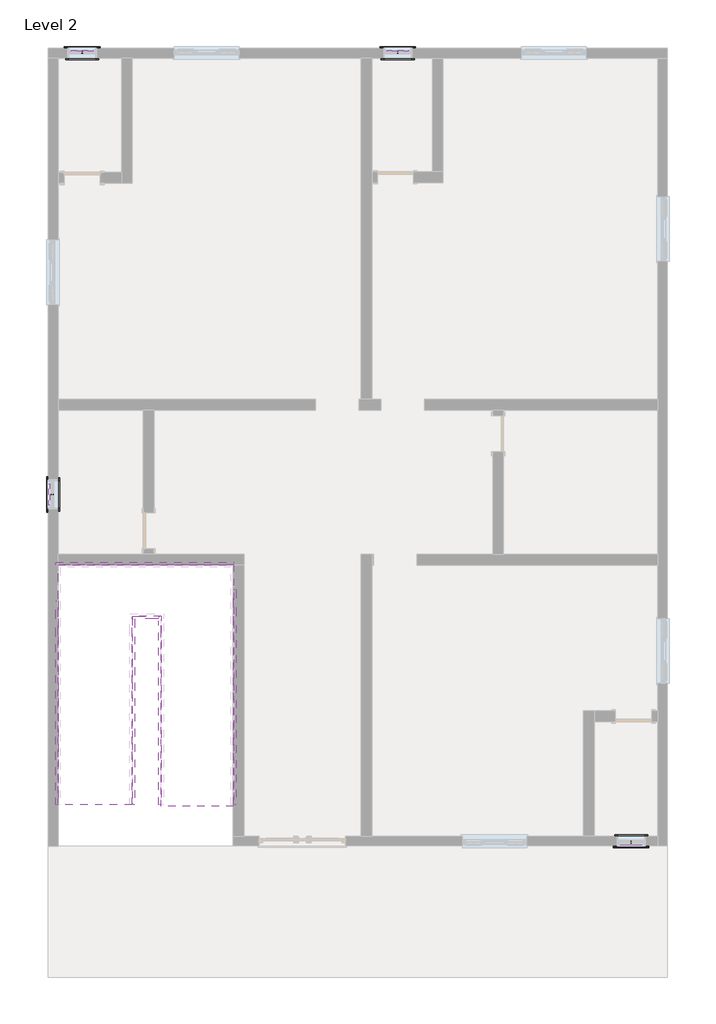
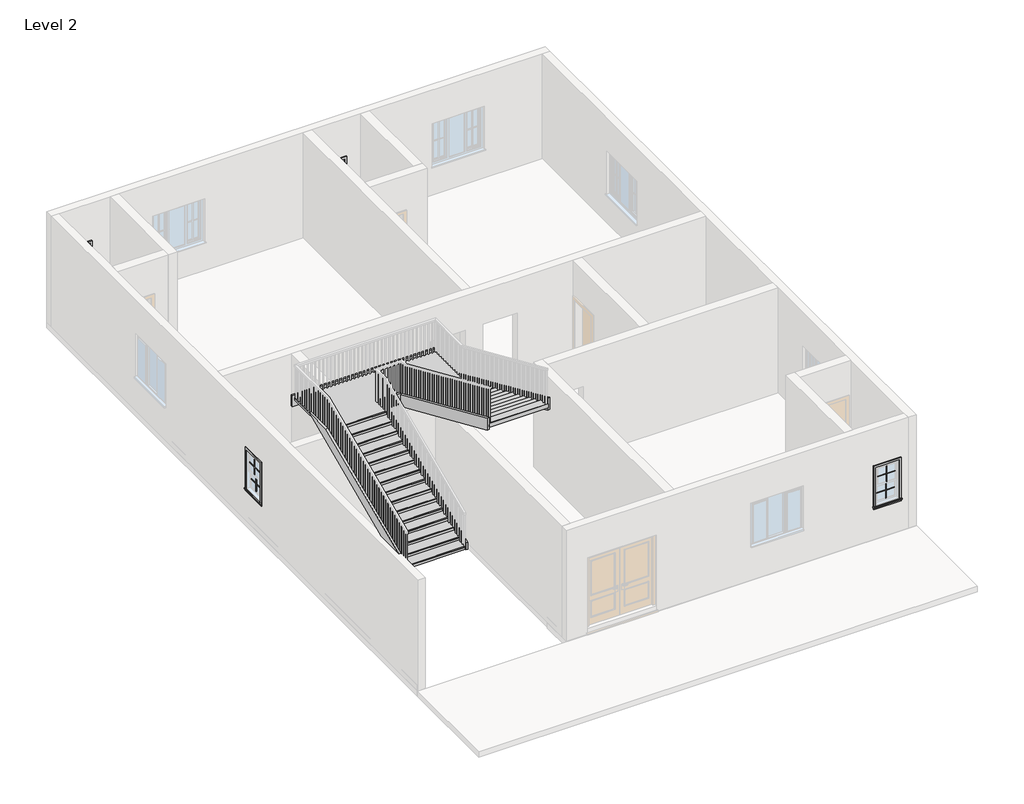
# One storey, part 4 of 4: 16 proxies, 6 members, 1 stair flight.
"""IFC4 building model written with IfcOpenShell, lengths in millimetres."""

from ifc_helpers import new_model, si_unit, frame, origin, place, context, project, spatial, polyline, outline, extrude, transform, mapped, element, save
from components import muntin_pattern_2x2_muntin_pattern_2x2_eba6c5fb, trim_window_exterior_flat_with_sill_278e6a94, trim_window_interior_flat_picture_frame_e9fd5f45, stair_flight_371d2c9c

model = new_model("IFC4")

# Units and contexts
model_context = context("Model", 3, world=origin())
ifc_project = project(units=[si_unit("LENGTHUNIT", "METRE", prefix="MILLI")], contexts=[model_context])

# Site, building, storey
site = spatial("IfcSite", under=ifc_project)
building = spatial("IfcBuilding", under=site)
storey = spatial("IfcBuildingStorey", under=building, Name="Level 2", Elevation=3048.0)

# Proxies
placement = place(None, origin())
muntin_pattern_2x2_muntin_pattern_2x2_shape = muntin_pattern_2x2_muntin_pattern_2x2_eba6c5fb(model_context)
element("IfcBuildingElementProxy", 1, Name="Muntin Pattern_2x2 : Muntin Pattern_2x2", ObjectType="Muntin Pattern_2x2 : Muntin Pattern_2x2", at=placement, inside=storey, context=model_context, shape_type="MappedRepresentation", body=[
    mapped(muntin_pattern_2x2_muntin_pattern_2x2_shape, transform((-7722.7165084, -455.2217109, 4518.025), x_axis=(0.0, 1.0, 0.0), y_axis=(-1.0, 0.0, 0.0), z_axis=(0.0, 0.0, 1.0))),
])
element("IfcBuildingElementProxy", 2, Name="Muntin Pattern_2x2 : Muntin Pattern_2x2", ObjectType="Muntin Pattern_2x2 : Muntin Pattern_2x2", at=placement, inside=storey, context=model_context, shape_type="MappedRepresentation", body=[
    mapped(muntin_pattern_2x2_muntin_pattern_2x2_shape, transform((-7678.2665084, -455.2217109, 4038.6), x_axis=(0.0, 1.0, 0.0), y_axis=(-1.0, 0.0, 0.0), z_axis=(0.0, 0.0, 1.0))),
])
element("IfcBuildingElementProxy", 3, Name="Muntin Pattern_2x2 : Muntin Pattern_2x2", ObjectType="Muntin Pattern_2x2 : Muntin Pattern_2x2", at=placement, inside=storey, context=model_context, shape_type="MappedRepresentation", body=[
    mapped(muntin_pattern_2x2_muntin_pattern_2x2_shape, transform((-7046.4415084, 8872.5685985, 4518.025), x_axis=(1.0, 0.0, 0.0), y_axis=(0.0, 1.0, 0.0), z_axis=(0.0, 0.0, 1.0))),
])
element("IfcBuildingElementProxy", 4, Name="Muntin Pattern_2x2 : Muntin Pattern_2x2", ObjectType="Muntin Pattern_2x2 : Muntin Pattern_2x2", at=placement, inside=storey, context=model_context, shape_type="MappedRepresentation", body=[
    mapped(muntin_pattern_2x2_muntin_pattern_2x2_shape, transform((-7046.4415084, 8828.1185985, 4038.6), x_axis=(1.0, 0.0, 0.0), y_axis=(0.0, 1.0, 0.0), z_axis=(0.0, 0.0, 1.0))),
])
element("IfcBuildingElementProxy", 5, Name="Muntin Pattern_2x2 : Muntin Pattern_2x2", ObjectType="Muntin Pattern_2x2 : Muntin Pattern_2x2", at=placement, inside=storey, context=model_context, shape_type="MappedRepresentation", body=[
    mapped(muntin_pattern_2x2_muntin_pattern_2x2_shape, transform((-417.0415084, 8872.5685985, 4518.025), x_axis=(1.0, 0.0, 0.0), y_axis=(0.0, 1.0, 0.0), z_axis=(0.0, 0.0, 1.0))),
])
element("IfcBuildingElementProxy", 6, Name="Muntin Pattern_2x2 : Muntin Pattern_2x2", ObjectType="Muntin Pattern_2x2 : Muntin Pattern_2x2", at=placement, inside=storey, context=model_context, shape_type="MappedRepresentation", body=[
    mapped(muntin_pattern_2x2_muntin_pattern_2x2_shape, transform((-417.0415084, 8828.1185985, 4038.6), x_axis=(1.0, 0.0, 0.0), y_axis=(0.0, 1.0, 0.0), z_axis=(0.0, 0.0, 1.0))),
])
element("IfcBuildingElementProxy", 7, Name="Muntin Pattern_2x2 : Muntin Pattern_2x2", ObjectType="Muntin Pattern_2x2 : Muntin Pattern_2x2", at=placement, inside=storey, context=model_context, shape_type="MappedRepresentation", body=[
    mapped(muntin_pattern_2x2_muntin_pattern_2x2_shape, transform((4485.1584916, -7796.1814015, 4518.025), x_axis=(-1.0, 0.0, 0.0), y_axis=(0.0, -1.0, 0.0), z_axis=(0.0, 0.0, 1.0))),
])
element("IfcBuildingElementProxy", 8, Name="Muntin Pattern_2x2 : Muntin Pattern_2x2", ObjectType="Muntin Pattern_2x2 : Muntin Pattern_2x2", at=placement, inside=storey, context=model_context, shape_type="MappedRepresentation", body=[
    mapped(muntin_pattern_2x2_muntin_pattern_2x2_shape, transform((4485.1584916, -7751.7314015, 4038.6), x_axis=(-1.0, 0.0, 0.0), y_axis=(0.0, -1.0, 0.0), z_axis=(0.0, 0.0, 1.0))),
])
trim_window_exterior_flat_with_sill_shape = trim_window_exterior_flat_with_sill_278e6a94(model_context)
element("IfcBuildingElementProxy", 9, Name="Trim-Window-Exterior-Flat : with Sill", ObjectType="Trim-Window-Exterior-Flat : with Sill", at=placement, inside=storey, context=model_context, shape_type="MappedRepresentation", body=[
    mapped(trim_window_exterior_flat_with_sill_shape, transform((-7757.6415084, -455.2217109, 5029.2), x_axis=(0.0, -1.0, 0.0), y_axis=(0.0, 0.0, 1.0), z_axis=(-1.0, 0.0, 0.0))),
])
element("IfcBuildingElementProxy", 10, Name="Trim-Window-Exterior-Flat : with Sill", ObjectType="Trim-Window-Exterior-Flat : with Sill", at=placement, inside=storey, context=model_context, shape_type="MappedRepresentation", body=[
    mapped(trim_window_exterior_flat_with_sill_shape, transform((-7046.4415084, 8907.4935985, 5029.2), x_axis=(-1.0, 0.0, 0.0), y_axis=(0.0, 0.0, 1.0), z_axis=(0.0, 1.0, 0.0))),
])
element("IfcBuildingElementProxy", 11, Name="Trim-Window-Exterior-Flat : with Sill", ObjectType="Trim-Window-Exterior-Flat : with Sill", at=placement, inside=storey, context=model_context, shape_type="MappedRepresentation", body=[
    mapped(trim_window_exterior_flat_with_sill_shape, transform((-417.0415084, 8907.4935985, 5029.2), x_axis=(-1.0, 0.0, 0.0), y_axis=(0.0, 0.0, 1.0), z_axis=(0.0, 1.0, 0.0))),
])
element("IfcBuildingElementProxy", 12, Name="Trim-Window-Exterior-Flat : with Sill", ObjectType="Trim-Window-Exterior-Flat : with Sill", at=placement, inside=storey, context=model_context, shape_type="MappedRepresentation", body=[
    mapped(trim_window_exterior_flat_with_sill_shape, transform((4485.1584916, -7831.1064015, 5029.2), x_axis=(1.0, 0.0, 0.0), y_axis=(0.0, 0.0, 1.0), z_axis=(0.0, -1.0, 0.0))),
])
trim_window_interior_flat_picture_frame_shape = trim_window_interior_flat_picture_frame_e9fd5f45(model_context)
element("IfcBuildingElementProxy", 13, Name="Trim-Window-Interior-Flat : Picture Frame", ObjectType="Trim-Window-Interior-Flat : Picture Frame", at=placement, inside=storey, context=model_context, shape_type="MappedRepresentation", body=[
    mapped(trim_window_interior_flat_picture_frame_shape, transform((-7554.4415084, -455.2217109, 5029.2), x_axis=(0.0, 1.0, 0.0), y_axis=(0.0, 0.0, 1.0), z_axis=(1.0, 0.0, 0.0))),
])
element("IfcBuildingElementProxy", 14, Name="Trim-Window-Interior-Flat : Picture Frame", ObjectType="Trim-Window-Interior-Flat : Picture Frame", at=placement, inside=storey, context=model_context, shape_type="MappedRepresentation", body=[
    mapped(trim_window_interior_flat_picture_frame_shape, transform((-7046.4415084, 8704.2935985, 5029.2), x_axis=(1.0, 0.0, 0.0), y_axis=(0.0, 0.0, 1.0), z_axis=(0.0, -1.0, 0.0))),
])
element("IfcBuildingElementProxy", 15, Name="Trim-Window-Interior-Flat : Picture Frame", ObjectType="Trim-Window-Interior-Flat : Picture Frame", at=placement, inside=storey, context=model_context, shape_type="MappedRepresentation", body=[
    mapped(trim_window_interior_flat_picture_frame_shape, transform((-417.0415084, 8704.2935985, 5029.2), x_axis=(1.0, 0.0, 0.0), y_axis=(0.0, 0.0, 1.0), z_axis=(0.0, -1.0, 0.0))),
])
element("IfcBuildingElementProxy", 16, Name="Trim-Window-Interior-Flat : Picture Frame", ObjectType="Trim-Window-Interior-Flat : Picture Frame", at=placement, inside=storey, context=model_context, shape_type="MappedRepresentation", body=[
    mapped(trim_window_interior_flat_picture_frame_shape, transform((4485.1584916, -7627.9064015, 5029.2), x_axis=(-1.0, 0.0, 0.0), y_axis=(0.0, 0.0, 1.0), z_axis=(0.0, 1.0, 0.0))),
])

# Members
element("IfcMember", 17, ObjectType="Stringer - 2\" Width", at=placement, inside=storey, context=model_context, shape_type="SweptSolid", body=[
    extrude(outline(polyline([(-6973.0610642, 5791.2), (-6973.0610642, 5990.0550815), (-3441.822613, 7543.8), (-2685.0041973, 7543.8), (-6668.1860155, 5791.2), (-6973.0610642, 5791.2)])), frame((-7605.2415084, 0.0, 0.0), z_axis=(1.0, 0.0, 0.0), x_axis=(0.0, 1.0, 0.0)), (0.0, 0.0, 1.0), 50.8),
])
element("IfcMember", 18, ObjectType="Stringer - 2\" Width", at=placement, inside=storey, context=model_context, shape_type="SweptSolid", body=[
    extrude(outline(polyline([(-7605.2415084, -1928.4217109), (-7605.2415084, -1877.6217109), (-3866.3290366, -1877.6217109), (-3866.3290366, -1928.4217109), (-7605.2415084, -1928.4217109)])), frame((0.0, 0.0, 7239.0), z_axis=(0.0, 0.0, 1.0), x_axis=(1.0, 0.0, 0.0)), (0.0, 0.0, 1.0), 304.8),
])
element("IfcMember", 19, ObjectType="Stringer - 2\" Width", at=placement, inside=storey, context=model_context, shape_type="SweptSolid", body=[
    extrude(outline(polyline([(-3202.3906584, 7239.0), (-6973.0610642, 8898.0949786), (-6973.0610642, 9231.0950815), (-2445.5722427, 7239.0), (-3202.3906584, 7239.0)])), frame((-3866.3290366, 0.0, 0.0), z_axis=(1.0, 0.0, 0.0), x_axis=(0.0, 1.0, 0.0)), (0.0, 0.0, 1.0), 50.8),
])
element("IfcMember", 20, ObjectType="Stringer - 2\" Width", at=placement, inside=storey, context=model_context, shape_type="SweptSolid", body=[
    extrude(outline(polyline([(-6973.0610642, 5791.2), (-6973.0610642, 5990.0550815), (-3441.822613, 7543.8), (-3061.4610642, 7543.8), (-3061.4610642, 7378.1589786), (-6668.1860155, 5791.2), (-6973.0610642, 5791.2)])), frame((-5999.9290366, 0.0, 0.0), z_axis=(1.0, 0.0, 0.0), x_axis=(0.0, 1.0, 0.0)), (0.0, 0.0, 1.0), 50.8),
])
element("IfcMember", 21, ObjectType="Stringer - 2\" Width", at=placement, inside=storey, context=model_context, shape_type="SweptSolid", body=[
    extrude(outline(polyline([(-5999.9290366, -3061.4610642), (-5999.9290366, -3010.6610642), (-5441.1290366, -3010.6610642), (-5441.1290366, -3061.4610642), (-5999.9290366, -3061.4610642)])), frame((0.0, 0.0, 7239.0), z_axis=(0.0, 0.0, 1.0), x_axis=(1.0, 0.0, 0.0)), (0.0, 0.0, 1.0), 304.8),
])
element("IfcMember", 22, ObjectType="Stringer - 2\" Width", at=placement, inside=storey, context=model_context, shape_type="SweptSolid", body=[
    extrude(outline(polyline([(-3010.6610642, 7487.6390815), (-3010.6610642, 7239.0), (-3202.3906584, 7239.0), (-6973.0610642, 8898.0949786), (-6973.0610642, 9231.0950815), (-3010.6610642, 7487.6390815)])), frame((-5441.1290366, 0.0, 0.0), z_axis=(1.0, 0.0, 0.0), x_axis=(0.0, 1.0, 0.0)), (0.0, 0.0, 1.0), 50.8),
])

# Stair flight
stair_flight_shape = stair_flight_371d2c9c(model_context)
element("IfcStairFlight", 23, ObjectType="2\" Tread 1\" Nosing 1/4\" Riser", at=placement, inside=storey, context=model_context, shape_type="MappedRepresentation", body=[
    mapped(stair_flight_shape, transform((0.0, 0.0, 0.0), x_axis=(1.0, 0.0, 0.0), y_axis=(0.0, 1.0, 0.0), z_axis=(0.0, 0.0, 1.0))),
])

save(model, "model.ifc")

# Revit data of these elements
# Type "Muntin Pattern_2x2 : Muntin Pattern_2x2"
#   Width [instance default] = 4' - 0"
#   Thickness = 0' - 0 1/2"
#   Height [instance default] = 4' - 0"
#   Distance = 0' - 0 3/4"
#   Interior Material [instance default] = none
#   Exterior Material [instance default] = none
#   Default Elevation = 0
# Type "Trim-Window-Exterior-Flat : with Sill"
#   Trim Width = 0' - 2 1/4"
#   Trim Thickness_Picture Frame = 0' - 1 1/4"
#   Trim Thickness_with Sill = 0' - 0 3/4"
#   Sill Thickness = 0' - 1 1/4"
#   Opening Width [instance default] = 2' - 0"
#   Opening Height [instance default] = 3' - 0"
#   Default Elevation = 4' - 0"
#   Sill = yes
#   Picture Frame = no
#   Trim Material [instance default] = none
# Type "Trim-Window-Interior-Flat : Picture Frame"
#   Trim Thickness_Picture Frame = 0' - 1 1/4"
#   Trim Width = 0' - 2 1/4"
#   Trim Thickness_with Sill = 0' - 0 3/4"
#   Sill Thickness = 0' - 1 1/4"
#   Opening Width [instance default] = 2' - 0"
#   Opening Height [instance default] = 3' - 0"
#   Default Elevation = 4' - 0"
#   Sill = no
#   Picture Frame = yes
#   Trim Material [instance default] = none
# Elements 1, 2, 3, 4, 5, 6, 7, 8 (IfcBuildingElementProxy, "Muntin Pattern_2x2 : Muntin Pattern_2x2")
#   Width = 1' - 6"
#   Height = 1' - 5 1/8"
#   Interior Material = Wood - Stained
#   Exterior Material = Clad - White
#   Phase Created = New Construction
#   Materials on its faces: "Clad - White", "Wood - Stained"
# Elements 9, 10, 11, 12 (IfcBuildingElementProxy, "Trim-Window-Exterior-Flat : with Sill")
#   Opening Width = 2' - 0"
#   Opening Height = 3' - 6"
#   Trim Material = Clad - White
#   Phase Created = New Construction
#   Materials on its faces: "Clad - White"
# Elements 13, 14, 15, 16 (IfcBuildingElementProxy, "Trim-Window-Interior-Flat : Picture Frame")
#   Opening Width = 2' - 0"
#   Opening Height = 3' - 6"
#   Trim Material = Wood - Stained
#   Phase Created = New Construction
#   Materials on its faces: "Wood - Stained"
# Elements 17, 18, 19, 20, 21, 22 (IfcMember, "Stringer - 2\" Width")
#   Phase Created = New Construction
# Element 23 (IfcStairFlight, "2\" Tread 1\" Nosing 1/4\" Riser")
#   Phase Created = New Construction
# Materials
#   "Clad - White": class "Wood", colour RGB 242 242 238, transparency 0, Cost = 0
#   "Wood - Stained": class "Wood", colour RGB 224 178 126, transparency 0, Cost = 0
